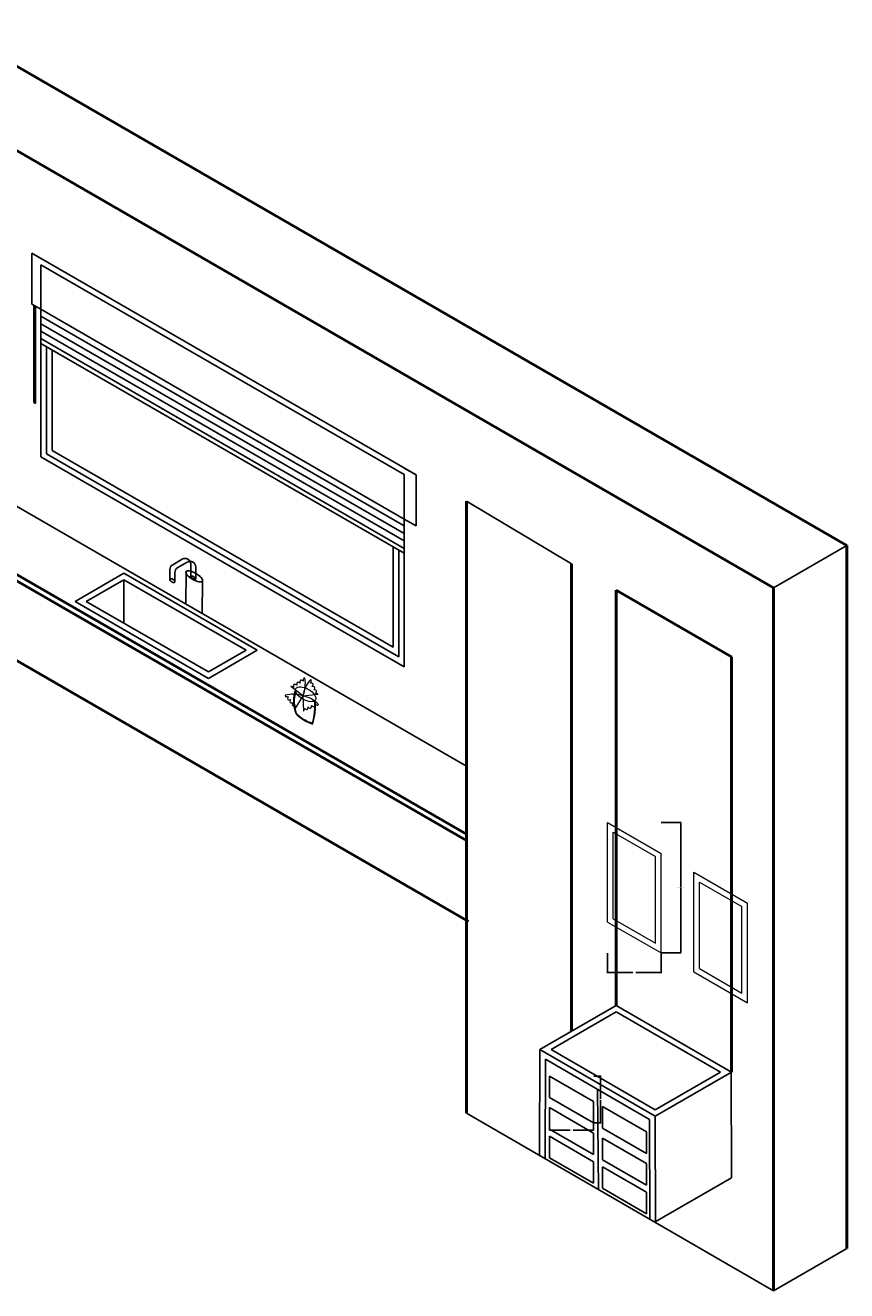
# Model space of a CAD drawing. Units: centimetres. Extents: x 16 to 604, y -284 to 166.
# Tile 2 of 2: x 312 to 604, y -284 to 166. Entities that reach past the tile are written whole.
import ezdxf

# ---------------------------------------------------------------- set-up
doc = ezdxf.new("R2010")
doc.units = ezdxf.units.CM
doc.header["$MEASUREMENT"] = 0
for name, color, linetype, lineweight in [('A-ANNO-DIMS', 2, 'Continuous', 18), ('A-FLOR-FIXT', 3, 'Continuous', 25), ('A-FURN-ACCS', 9, 'Continuous', 18), ('A-FURN-CASE', 8, 'Continuous', 25), ('A-GLAZ', 4, 'Continuous', 25), ('A-WALL', 7, 'Continuous', 50)]:
    doc.layers.add(name, color=color, linetype=linetype, lineweight=lineweight)
doc.styles.get("Standard").update_dxf_attribs({"font": 'arial.ttf'})
doc.dimstyles.get("Standard").update_dxf_attribs({"dimtxt": 0.18, "dimasz": 0.18, "dimexe": 0.18, "dimexo": 0.0625, "dimgap": 0.09, "dimtad": 0, "dimtih": 1, "dimtoh": 1, "dimdec": 0, "dimzin": 0, "dimdsep": 46, "dimtxsty": 'Standard', "dimcen": 0.09, "dimadec": 0, "dimazin": 0, "dimtfac": 1, "dimtdec": 0, "dimtofl": 0, "dimtmove": 0, "dimatfit": 3, "dimfxl": 1, "dimtolj": 1, "dimtzin": 0, "dimarcsym": 0})

# ---------------------------------------------------------------- blocks, each defined once
blk = doc.blocks.new('PICTURE-FRAME')
for p, q in [((0, 11), (0, 46.42)), ((0, 46.42), (19.05, 35.42)), ((2, 12.15), (2, 42.96)), ((2, 42.96), (17.05, 34.27)), ((17.05, 3.46), (17.05, 34.27)), ((19.05, 0), (19.05, 35.42)), ((0, 11), (19.05, 0)), ((2, 12.15), (17.05, 3.46))]:
    blk.add_line(p, q)
blk = doc.blocks.new('DRAWER-FRONT')
for p, q in [((0, 16.69), (15.64, 7.66)), ((0, 16.69), (0, 9.03)), ((0, 9.03), (15.64, 0)), ((15.64, 7.66), (15.64, 0))]:
    blk.add_line(p, q)
blk = doc.blocks.new('*D11')
at = {"layer": 'A-ANNO-DIMS', "color": 0, "lineweight": -2, "transparency": 16777216}
for p, q in [((514.52, -207.25), (517.14, -207.25)), ((516.96, -207.43), (516.96, -215.41)), ((516.96, -223.76), (516.96, -215.78)), ((514.52, -223.94), (517.14, -223.94))]:
    blk.add_line(p, q, dxfattribs=at)
at = {"layer": 'A-ANNO-DIMS', "color": 0, "transparency": 16777216}
for points in [[(516.93, -207.43), (516.99, -207.43), (516.96, -207.25)], [(516.93, -223.76), (516.99, -223.76), (516.96, -223.94)]]:
    blk.add_solid(points, dxfattribs=at)
at = {"layer": 'Defpoints', "color": 0, "transparency": 16777216}
for p in [(514.45, -207.25), (516.96, -207.25), (514.45, -223.94)]:
    blk.add_point(p, dxfattribs=at)
at = {"layer": 'A-ANNO-DIMS', "color": 0, "transparency": 16777216, "insert": (516.96, -215.6), "char_height": 0.18, "attachment_point": 5}
blk.add_mtext('\\A1;DRAWER FRONT 17 TYP.', dxfattribs=at)
blk = doc.blocks.new('*D12')
at = {"layer": 'A-ANNO-DIMS', "color": 0, "lineweight": -2, "transparency": 16777216}
for p, q in [((498.81, -224), (498.81, -226.62)), ((514.45, -224), (514.45, -226.62)), ((498.99, -226.44), (506.11, -226.44)), ((514.27, -226.44), (507.15, -226.44))]:
    blk.add_line(p, q, dxfattribs=at)
at = {"layer": 'A-ANNO-DIMS', "color": 0, "transparency": 16777216}
for points in [[(498.99, -226.41), (498.99, -226.47), (498.81, -226.44)], [(514.27, -226.41), (514.27, -226.47), (514.45, -226.44)]]:
    blk.add_solid(points, dxfattribs=at)
at = {"layer": 'Defpoints', "color": 0, "transparency": 16777216}
for p in [(498.81, -223.94), (514.45, -223.94), (514.45, -226.44)]:
    blk.add_point(p, dxfattribs=at)
at = {"layer": 'A-ANNO-DIMS', "color": 0, "transparency": 16777216, "insert": (506.63, -226.44), "char_height": 0.18, "attachment_point": 5}
blk.add_mtext('\\A1;16 TYP.', dxfattribs=at)
blk = doc.blocks.new('*D19')
at = {"layer": 'A-ANNO-DIMS', "color": 0, "lineweight": -2, "transparency": 16777216}
for p, q in [((538.54, -117.06), (545.62, -117.06)), ((545.44, -117.24), (545.44, -140.09)), ((545.44, -163.3), (545.44, -140.46)), ((538.54, -163.48), (545.62, -163.48))]:
    blk.add_line(p, q, dxfattribs=at)
at = {"layer": 'A-ANNO-DIMS', "color": 0, "transparency": 16777216}
for points in [[(545.41, -117.24), (545.47, -117.24), (545.44, -117.06)], [(545.41, -163.3), (545.47, -163.3), (545.44, -163.48)]]:
    blk.add_solid(points, dxfattribs=at)
at = {"layer": 'Defpoints', "color": 0, "transparency": 16777216}
for p in [(538.48, -117.06), (545.44, -117.06), (538.48, -163.48)]:
    blk.add_point(p, dxfattribs=at)
at = {"layer": 'A-ANNO-DIMS', "color": 0, "transparency": 16777216, "insert": (545.44, -140.27), "char_height": 0.18, "attachment_point": 5}
blk.add_mtext('\\A1;PICTURE FRAME 46 TYP.', dxfattribs=at)
blk = doc.blocks.new('*D20')
at = {"layer": 'A-ANNO-DIMS', "color": 0, "lineweight": -2, "transparency": 16777216}
for p, q in [((519.43, -163.55), (519.43, -170.63)), ((538.48, -163.55), (538.48, -170.63)), ((519.61, -170.45), (528.43, -170.45)), ((538.3, -170.45), (529.47, -170.45))]:
    blk.add_line(p, q, dxfattribs=at)
at = {"layer": 'A-ANNO-DIMS', "color": 0, "transparency": 16777216}
for points in [[(519.61, -170.42), (519.61, -170.48), (519.43, -170.45)], [(538.3, -170.42), (538.3, -170.48), (538.48, -170.45)]]:
    blk.add_solid(points, dxfattribs=at)
at = {"layer": 'Defpoints', "color": 0, "transparency": 16777216}
for p in [(519.43, -163.48), (538.48, -163.48), (538.48, -170.45)]:
    blk.add_point(p, dxfattribs=at)
at = {"layer": 'A-ANNO-DIMS', "color": 0, "transparency": 16777216, "insert": (528.95, -170.45), "char_height": 0.18, "attachment_point": 5}
blk.add_mtext('\\A1;19 TYP.', dxfattribs=at)

msp = doc.modelspace()

# ---------------------------------------------------------------- linework, layer by layer
at = {"layer": 'A-FLOR-FIXT'}
for p, q in [((445.15, -58.22), (319.94, 14.07)), ((447.15, -61.68), (317.94, 12.92)), ((299.16, 1.14), (469.25, -97.06)), ((368.2, -23.46), (364.79, -25.43)), ((369.98, -24.48), (366.57, -26.45)), ((371.2, -29.5), (371.2, -25.19)), ((372.98, -30.52), (372.98, -26.21)), ((347.44, -28.46), (330.06, -38.49)), ((347.44, -30.77), (334.06, -38.49)), ((394.86, -55.84), (347.44, -28.46)), ((390.86, -55.84), (347.44, -30.77)), ((347.44, -30.77), (347.44, -46.22)), ((363.79, -27.16), (363.79, -30.57)), ((365.57, -28.18), (365.57, -31.6)), ((369.47, -39.45), (369.54, -27.85)), ((375.3, -42.81), (375.37, -31.21)), ((330.06, -38.49), (377.48, -65.87)), ((334.06, -38.49), (377.48, -63.56)), ((377.48, -65.87), (394.86, -55.84)), ((377.48, -63.56), (390.86, -55.84))]:
    msp.add_line(p, q, dxfattribs=at)
for centre, start, end in [((365.79, -27.16), 120, 180), ((367.57, -28.18), 120, 180), ((369.2, -25.19), 0, 120), ((370.98, -26.21), 0, 120)]:
    msp.add_arc(centre, 2, start, end, dxfattribs=at)
for centre, major_axis, ratio in [((364.68, -31.08), (-0.887, 0.512), 0.5), ((372.45, -29.53), (-2.91, 1.68), 0.353341), ((372.09, -30.01), (-0.887, 0.512), 0.341621)]:
    msp.add_ellipse(centre, major_axis=major_axis, ratio=ratio, dxfattribs=at)
at = {"layer": 'A-FURN-ACCS'}
for q in [(406.77, -68.76), (416.53, -71.45), (408.17, -76.61), (411.31, -77.47)]:
    msp.add_line((411.12, -72.03), q, dxfattribs=at)
for centre, radius, start, end in [((410.04, -67.93), 1.17, 145.1386, 197.4091), ((409.29, -68.41), 1.17, 48.4851, 100.7555), ((411.19, -67.18), 1.17, 145.1386, 197.4091), ((410.45, -67.67), 1.17, 48.4851, 100.7555), ((400.43, -67.71), 11.53, 337.9889, 9.7154), ((422.51, -73.8), 11.53, 139.4559, 171.1823), ((412.34, -66.44), 1.17, 145.1386, 197.4091), ((411.6, -66.92), 1.17, 80.4513, 100.7555), ((412.93, -66.6), 1.17, 311.7622, 4.0326), ((413.93, -68.63), 1.17, 48.4157, 100.6862), ((413.32, -67.39), 1.17, 48.4157, 68.72), ((405.99, -71.92), 1.17, 174.6444, 194.9487), ((407.59, -83.01), 11.53, 72.1821, 103.9085), ((406.99, -69.91), 1.17, 48.4851, 100.7555), ((408.88, -68.68), 1.17, 145.1386, 197.4091), ((419.81, -73.92), 12.08, 159.9827, 201.5759), ((408.14, -69.16), 1.17, 48.4851, 100.7555), ((420.07, -74.18), 12.08, 162.7463, 199.6173), ((413.54, -67.83), 1.17, 311.7622, 4.0326), ((414.54, -69.86), 1.17, 48.4157, 100.6862), ((414.15, -69.07), 1.17, 311.7622, 4.0326), ((415.15, -71.09), 1.17, 48.4157, 100.6862), ((414.75, -70.3), 1.17, 311.7622, 4.0326), ((415.75, -72.33), 1.17, 48.4157, 100.6862), ((405.45, -71.22), 1.17, 239.3318, 291.6022), ((406.82, -73.02), 1.17, 142.6782, 194.9487), ((406.28, -72.31), 1.17, 239.3318, 291.6022), ((407.65, -74.11), 1.17, 142.6782, 194.9487), ((407.11, -73.41), 1.17, 239.3318, 291.6022), ((408.48, -75.21), 1.17, 142.6782, 194.9487), ((407.94, -74.5), 1.17, 239.3318, 291.6022), ((409.3, -76.31), 1.17, 142.6782, 194.9487), ((408.54, -83.27), 11.53, 45.3675, 77.0939), ((410.49, -76.63), 1.17, 314.3274, 6.5978), ((412.59, -75.78), 1.17, 217.6738, 269.9442), ((411.77, -76.11), 1.17, 314.3274, 6.5978), ((413.86, -75.26), 1.17, 217.6738, 269.9442), ((413.04, -75.6), 1.17, 314.3274, 6.5978), ((415.13, -74.74), 1.17, 217.6738, 269.9442), ((396.52, -75.88), 18.85, 341.8327, 6.4065), ((396.77, -75.58), 18.85, 339.9033, 6.4065), ((414.31, -75.08), 1.17, 314.3274, 6.5978), ((416.4, -74.23), 1.17, 217.6738, 269.9442), ((415.58, -74.56), 1.17, 314.3274, 334.6316), ((419.19, -67.98), 14.85, 224.3647, 251.4899), ((419.13, -67.67), 14.85, 225.323, 251.5352)]:
    msp.add_arc(centre, radius, start, end, dxfattribs=at)
msp.add_ellipse((412.05, -71.48), major_axis=(-3.47, 2), ratio=0.501826, dxfattribs=at)
at = {"layer": 'A-FURN-CASE'}
for p, q in [((469.25, -2.85), (506.63, -25.05)), ((604.48, -18.59), (578.5, -33.59)), ((522.51, -182.14), (495.34, -197.82)), ((522.51, -184.45), (499.34, -197.82)), ((522.51, -182.14), (563.56, -205.83)), ((522.51, -184.45), (559.56, -205.83)), ((495.34, -197.82), (495.25, -235.52)), ((536.38, -221.52), (495.34, -197.82)), ((536.38, -219.21), (499.34, -197.82)), ((497.33, -201.28), (497.25, -236.68)), ((534.39, -222.68), (497.33, -201.28)), ((563.56, -205.83), (536.38, -221.52)), ((559.56, -205.83), (536.38, -219.21)), ((563.37, -205.94), (563.49, -243.48)), ((515.86, -211.98), (516.19, -247.62)), ((578.5, -283.59), (469.25, -220.51)), ((534.39, -222.68), (534.5, -258.19)), ((536.38, -221.52), (536.51, -259.34)), ((563.49, -243.48), (536.38, -259.13)), ((604.48, -268.59), (578.5, -283.59))]:
    msp.add_line(p, q, dxfattribs=at)
at = {"layer": 'A-GLAZ'}
for p, q in [((314.7, 85.41), (451.31, 6.54)), ((314.7, 67.29), (314.7, 85.41)), ((314.7, 85.41), (317.94, 83.54)), ((317.94, 81.23), (447.15, 6.63)), ((317.94, 65.42), (317.94, 81.23)), ((317.94, 65.42), (314.7, 67.29)), ((315.35, 66.91), (315.35, 32.24)), ((316, 66.54), (316, 31.87)), ((317.94, 65.42), (447.15, -9.18)), ((317.94, 65.42), (317.94, 53.26)), ((317.94, 62.96), (447.15, -11.64)), ((317.94, 60.29), (447.15, -14.31)), ((317.94, 57.67), (447.15, -16.93)), ((317.94, 55), (447.15, -19.6)), ((317.94, 12.92), (317.94, 53.26)), ((317.94, 53.26), (447.15, -21.33)), ((319.94, 14.07), (319.94, 52.11)), ((321.94, 15.23), (321.94, 50.96)), ((315.35, 32.24), (316, 31.87)), ((443.15, -54.75), (321.94, 15.23)), ((451.31, 6.54), (447.15, 8.94)), ((447.15, 6.63), (447.15, -9.18)), ((451.31, -11.58), (451.31, 6.54)), ((447.15, -9.18), (447.15, -21.33)), ((447.15, -9.18), (451.31, -11.58)), ((443.15, -19.02), (443.15, -54.75)), ((445.15, -20.18), (445.15, -58.22)), ((447.15, -21.33), (447.15, -61.68))]:
    msp.add_line(p, q, dxfattribs=at)
at = {"layer": 'A-WALL'}
for p, q in [((284.05, 166.41), (604.48, -18.59)), ((578.5, -33.59), (258.07, 151.41)), ((469.25, -220.51), (469.25, -2.85)), ((604.48, -18.59), (604.48, -268.59)), ((299.95, -23.47), (469.25, -121.22)), ((299.95, -23.47), (469.25, -121.22)), ((299.95, -25.78), (469.25, -123.52)), ((506.63, -191.31), (506.63, -25.05)), ((522.51, -34.48), (522.51, -182.14)), ((522.51, -34.48), (563.56, -58.18)), ((578.5, -283.59), (578.5, -33.59)), ((299.95, -54.11), (470.03, -152.31)), ((563.56, -58.18), (563.56, -205.83))]:
    msp.add_line(p, q, dxfattribs=at)

# ---------------------------------------------------------------- block references
at = {"layer": 'A-FURN-ACCS'}
for p in [(519.43, -163.49), (550.13, -181.21)]:
    msp.add_blockref('PICTURE-FRAME', p, dxfattribs=at)
at = {"layer": 'A-FURN-CASE'}
for p in [(498.81, -223.94), (498.81, -235.17), (517.6, -234.79), (498.81, -245.37), (517.6, -246.02), (517.6, -256.21)]:
    msp.add_blockref('DRAWER-FRONT', p, dxfattribs=at)

# ---------------------------------------------------------------- dimensions: what is measured, and where the dimension line sits
at = {"layer": 'A-ANNO-DIMS'}
for base, p1, p2, text, picture, middle in [((545.44, -117.06), (538.48, -163.49), (538.48, -117.06), 'PICTURE FRAME <> TYP.', '*D19', (545.44, -140.27)), ((516.96, -207.25), (514.45, -223.94), (514.45, -207.25), 'DRAWER FRONT <> TYP.', '*D11', (516.96, -215.6))]:
    dim = msp.add_linear_dim(base=base, p1=p1, p2=p2, angle=90, text=text, dimstyle='Standard', override={"dimdec": 0, "dimlfac": 1, "dimrnd": 0, "dimzin": 0, "dimdsep": 46, "dimlunit": 2}, dxfattribs=at)
    dim.commit()
    dim.dimension.update_dxf_attribs({"geometry": picture, "text_midpoint": middle})
for base, p1, p2, picture, middle in [((538.48, -170.45), (519.43, -163.49), (538.48, -163.49), '*D20', (528.95, -170.45)), ((514.45, -226.44), (498.81, -223.94), (514.45, -223.94), '*D12', (506.63, -226.44))]:
    dim = msp.add_linear_dim(base=base, p1=p1, p2=p2, text='<> TYP.', dimstyle='Standard', override={"dimdec": 0, "dimlfac": 1, "dimrnd": 0, "dimzin": 0, "dimdsep": 46, "dimlunit": 2}, dxfattribs=at)
    dim.commit()
    dim.dimension.update_dxf_attribs({"geometry": picture, "text_midpoint": middle})

doc.saveas('drawing.dxf')
